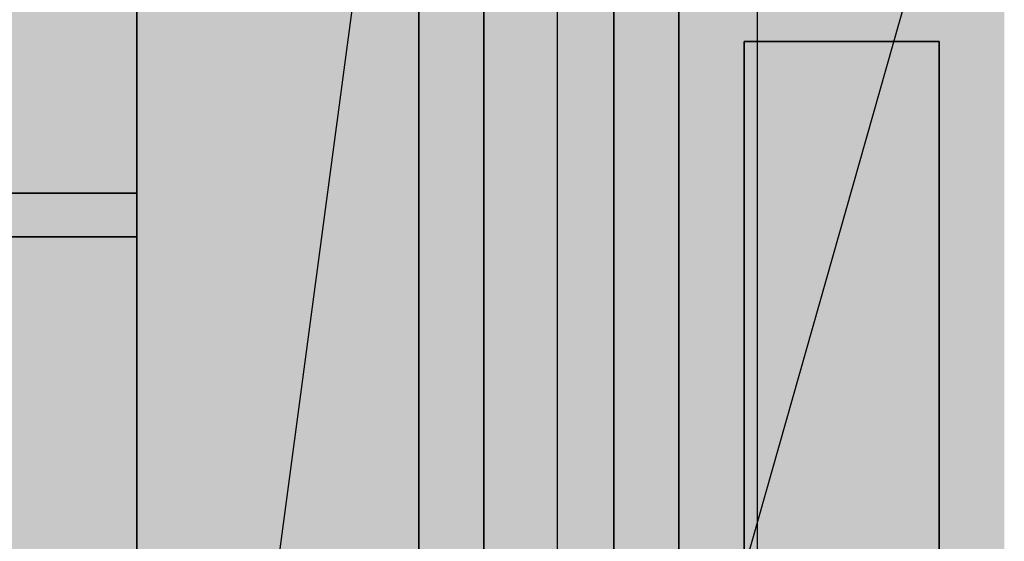
# Model space of a CAD drawing. Units: millimetres. Extents: x 130 to 1021, y 147 to 699.
# Tile 28 of 40: x 442 to 487, y 524 to 548. Entities that reach past the tile are written whole.
import ezdxf

# ---------------------------------------------------------------- set-up
doc = ezdxf.new("R2010")
doc.units = ezdxf.units.MM
doc.header["$MEASUREMENT"] = 0
for name, color, linetype, lineweight in [('A-ANNO-DIMS', 2, 'Continuous', 18), ('A-ELEV', 7, 'Continuous', 35), ('A-ELEV-PATT', 9, 'Continuous', 13)]:
    doc.layers.add(name, color=color, linetype=linetype, lineweight=lineweight)
doc.styles.get("Standard").update_dxf_attribs({"font": 'arial.ttf'})
doc.dimstyles.get("Standard").update_dxf_attribs({"dimtxt": 20, "dimasz": 10, "dimexe": 10, "dimexo": 10, "dimgap": 5, "dimtad": 0, "dimtih": 1, "dimtoh": 1, "dimdec": 0, "dimzin": 0, "dimdsep": 46, "dimtxsty": 'Standard', "dimcen": 5, "dimadec": 0, "dimazin": 0, "dimtfac": 1, "dimtdec": 0, "dimtofl": 0, "dimtmove": 0, "dimatfit": 3, "dimfxl": 1, "dimtolj": 1, "dimtzin": 0, "dimarcsym": 0})

# ---------------------------------------------------------------- blocks, each defined once
blk = doc.blocks.new('*D11')
at = {"layer": 'A-ANNO-DIMS', "color": 0, "lineweight": -2, "transparency": 16777216}
for p, q in [((737.374, 648.699), (737.374, 149.739)), ((299.374, 566.947), (299.374, 149.739)), ((309.374, 159.739), (490.857, 159.739)), ((727.374, 159.739), (545.891, 159.739))]:
    blk.add_line(p, q, dxfattribs=at)
at = {"layer": 'A-ANNO-DIMS', "color": 0, "transparency": 16777216}
for points in [[(309.374, 161.406), (309.374, 158.073), (299.374, 159.739)], [(727.374, 161.406), (727.374, 158.073), (737.374, 159.739)]]:
    blk.add_solid(points, dxfattribs=at)
at = {"layer": 'Defpoints', "color": 0, "transparency": 16777216}
for p in [(737.374, 658.699), (299.374, 576.947), (737.374, 159.739)]:
    blk.add_point(p, dxfattribs=at)
at = {"layer": 'A-ANNO-DIMS', "color": 0, "transparency": 16777216, "insert": (518.374, 159.739), "char_height": 20, "attachment_point": 5}
blk.add_mtext('\\A1;438', dxfattribs=at)
blk = doc.blocks.new('*D12')
at = {"layer": 'A-ANNO-DIMS', "color": 0, "lineweight": -2, "transparency": 16777216}
for p, q in [((477.374, 661.947), (265.074, 661.947)), ((275.074, 651.947), (275.074, 438.205)), ((275.074, 194.039), (275.074, 407.782)), ((357.163, 184.039), (265.074, 184.039))]:
    blk.add_line(p, q, dxfattribs=at)
at = {"layer": 'A-ANNO-DIMS', "color": 0, "transparency": 16777216}
for points in [[(273.407, 651.947), (276.74, 651.947), (275.074, 661.947)], [(273.407, 194.039), (276.74, 194.039), (275.074, 184.039)]]:
    blk.add_solid(points, dxfattribs=at)
at = {"layer": 'Defpoints', "color": 0, "transparency": 16777216}
for p in [(275.074, 661.947), (487.374, 661.947), (367.163, 184.039)]:
    blk.add_point(p, dxfattribs=at)
at = {"layer": 'A-ANNO-DIMS', "color": 0, "transparency": 16777216, "insert": (275.074, 422.993), "char_height": 20, "attachment_point": 5}
blk.add_mtext('\\A1;477.9', dxfattribs=at)
blk = doc.blocks.new('*D16')
at = {"layer": 'A-ANNO-DIMS', "color": 0, "lineweight": -2, "transparency": 16777216}
for p, q in [((357.941, 411.947), (357.941, 696.247)), ((363.922, 579.884), (363.922, 696.247)), ((347.941, 686.247), (337.941, 686.247)), ((373.922, 686.247), (383.922, 686.247))]:
    blk.add_line(p, q, dxfattribs=at)
at = {"layer": 'A-ANNO-DIMS', "color": 0, "transparency": 16777216}
for points in [[(347.941, 687.914), (347.941, 684.581), (357.941, 686.247)], [(373.922, 687.914), (373.922, 684.581), (363.922, 686.247)]]:
    blk.add_solid(points, dxfattribs=at)
at = {"layer": 'Defpoints', "color": 0, "transparency": 16777216}
for p in [(363.922, 686.247), (363.922, 569.884), (357.941, 401.947)]:
    blk.add_point(p, dxfattribs=at)
at = {"layer": 'A-ANNO-DIMS', "color": 0, "transparency": 16777216, "insert": (420.737, 686.247), "char_height": 20, "attachment_point": 5}
blk.add_mtext('\\A1;5.981', dxfattribs=at)
blk = doc.blocks.new('*D17')
at = {"layer": 'A-ANNO-DIMS', "color": 0, "lineweight": -2, "transparency": 16777216}
for p, q in [((363.922, 579.884), (363.922, 696.247)), ((375.85, 490.216), (375.85, 696.247)), ((353.922, 686.247), (343.922, 686.247)), ((385.85, 686.247), (395.85, 686.247))]:
    blk.add_line(p, q, dxfattribs=at)
at = {"layer": 'A-ANNO-DIMS', "color": 0, "transparency": 16777216}
for points in [[(353.922, 687.914), (353.922, 684.581), (363.922, 686.247)], [(385.85, 687.914), (385.85, 684.581), (375.85, 686.247)]]:
    blk.add_solid(points, dxfattribs=at)
at = {"layer": 'Defpoints', "color": 0, "transparency": 16777216}
for p in [(375.85, 686.247), (363.922, 569.884), (375.85, 480.216)]:
    blk.add_point(p, dxfattribs=at)
at = {"layer": 'A-ANNO-DIMS', "color": 0, "transparency": 16777216, "insert": (441.444, 686.247), "char_height": 20, "attachment_point": 5}
blk.add_mtext('\\A1;11.928', dxfattribs=at)
blk = doc.blocks.new('*D18')
at = {"layer": 'A-ANNO-DIMS', "color": 0, "lineweight": -2, "transparency": 16777216}
for p, q in [((375.85, 490.216), (375.85, 696.247)), ((382.374, 388.947), (382.374, 696.247)), ((365.85, 686.247), (355.85, 686.247)), ((392.374, 686.247), (402.374, 686.247))]:
    blk.add_line(p, q, dxfattribs=at)
at = {"layer": 'A-ANNO-DIMS', "color": 0, "transparency": 16777216}
for points in [[(365.85, 687.914), (365.85, 684.581), (375.85, 686.247)], [(392.374, 687.914), (392.374, 684.581), (382.374, 686.247)]]:
    blk.add_solid(points, dxfattribs=at)
at = {"layer": 'Defpoints', "color": 0, "transparency": 16777216}
for p in [(382.374, 686.247), (375.85, 480.216), (382.374, 378.947)]:
    blk.add_point(p, dxfattribs=at)
at = {"layer": 'A-ANNO-DIMS', "color": 0, "transparency": 16777216, "insert": (441.132, 686.247), "char_height": 20, "attachment_point": 5}
blk.add_mtext('\\A1;6.524', dxfattribs=at)
blk = doc.blocks.new('*D19')
at = {"layer": 'A-ANNO-DIMS', "color": 0, "lineweight": -2, "transparency": 16777216}
for p, q in [((382.374, 388.947), (382.374, 696.247)), ((414.652, 510.881), (414.652, 696.247)), ((392.374, 686.247), (404.652, 686.247)), ((414.652, 686.247), (424.652, 686.247))]:
    blk.add_line(p, q, dxfattribs=at)
at = {"layer": 'A-ANNO-DIMS', "color": 0, "transparency": 16777216}
for points in [[(392.374, 687.914), (392.374, 684.581), (382.374, 686.247)], [(404.652, 687.914), (404.652, 684.581), (414.652, 686.247)]]:
    blk.add_solid(points, dxfattribs=at)
at = {"layer": 'Defpoints', "color": 0, "transparency": 16777216}
for p in [(414.652, 686.247), (414.652, 500.881), (382.374, 378.947)]:
    blk.add_point(p, dxfattribs=at)
at = {"layer": 'A-ANNO-DIMS', "color": 0, "transparency": 16777216, "insert": (463.411, 686.247), "char_height": 20, "attachment_point": 5}
blk.add_mtext('\\A1;32.28', dxfattribs=at)
blk = doc.blocks.new('*D20')
at = {"layer": 'A-ANNO-DIMS', "color": 0, "lineweight": -2, "transparency": 16777216}
for p, q in [((414.652, 510.881), (414.652, 696.247)), ((432.374, 388.947), (432.374, 696.247)), ((404.652, 686.247), (394.652, 686.247)), ((442.374, 686.247), (452.374, 686.247))]:
    blk.add_line(p, q, dxfattribs=at)
at = {"layer": 'A-ANNO-DIMS', "color": 0, "transparency": 16777216}
for points in [[(404.652, 687.914), (404.652, 684.581), (414.652, 686.247)], [(442.374, 687.914), (442.374, 684.581), (432.374, 686.247)]]:
    blk.add_solid(points, dxfattribs=at)
at = {"layer": 'Defpoints', "color": 0, "transparency": 16777216}
for p in [(432.374, 686.247), (414.652, 500.881), (432.374, 378.947)]:
    blk.add_point(p, dxfattribs=at)
at = {"layer": 'A-ANNO-DIMS', "color": 0, "transparency": 16777216, "insert": (490.075, 686.247), "char_height": 20, "attachment_point": 5}
blk.add_mtext('\\A1;17.72', dxfattribs=at)
blk = doc.blocks.new('*D21')
at = {"layer": 'A-ANNO-DIMS', "color": 0, "lineweight": -2, "transparency": 16777216}
for p, q in [((432.374, 388.947), (432.374, 696.247)), ((447.374, 656.947), (447.374, 696.247)), ((422.374, 686.247), (412.374, 686.247)), ((457.374, 686.247), (467.374, 686.247))]:
    blk.add_line(p, q, dxfattribs=at)
at = {"layer": 'A-ANNO-DIMS', "color": 0, "transparency": 16777216}
for points in [[(422.374, 687.914), (422.374, 684.581), (432.374, 686.247)], [(457.374, 687.914), (457.374, 684.581), (447.374, 686.247)]]:
    blk.add_solid(points, dxfattribs=at)
at = {"layer": 'Defpoints', "color": 0, "transparency": 16777216}
for p in [(447.374, 686.247), (447.374, 646.947), (432.374, 378.947)]:
    blk.add_point(p, dxfattribs=at)
at = {"layer": 'A-ANNO-DIMS', "color": 0, "transparency": 16777216, "insert": (485.832, 686.247), "char_height": 20, "attachment_point": 5}
blk.add_mtext('\\A1;15', dxfattribs=at)
blk = doc.blocks.new('*D22')
at = {"layer": 'A-ANNO-DIMS', "color": 0, "lineweight": -2, "transparency": 16777216}
for p, q in [((447.374, 656.947), (447.374, 696.247)), ((466.767, 403.947), (466.767, 696.247)), ((437.374, 686.247), (427.374, 686.247)), ((476.767, 686.247), (486.767, 686.247))]:
    blk.add_line(p, q, dxfattribs=at)
at = {"layer": 'A-ANNO-DIMS', "color": 0, "transparency": 16777216}
for points in [[(437.374, 687.914), (437.374, 684.581), (447.374, 686.247)], [(476.767, 687.914), (476.767, 684.581), (466.767, 686.247)]]:
    blk.add_solid(points, dxfattribs=at)
at = {"layer": 'Defpoints', "color": 0, "transparency": 16777216}
for p in [(466.767, 686.247), (447.374, 646.947), (466.767, 393.947)]:
    blk.add_point(p, dxfattribs=at)
at = {"layer": 'A-ANNO-DIMS', "color": 0, "transparency": 16777216, "insert": (532.34, 686.247), "char_height": 20, "attachment_point": 5}
blk.add_mtext('\\A1;19.393', dxfattribs=at)
blk = doc.blocks.new('*D23')
at = {"layer": 'A-ANNO-DIMS', "color": 0, "lineweight": -2, "transparency": 16777216}
for p, q in [((466.767, 403.947), (466.767, 696.247)), ((475.988, 209.039), (475.988, 696.247)), ((456.767, 686.247), (446.767, 686.247)), ((485.988, 686.247), (495.988, 686.247))]:
    blk.add_line(p, q, dxfattribs=at)
at = {"layer": 'A-ANNO-DIMS', "color": 0, "transparency": 16777216}
for points in [[(456.767, 687.914), (456.767, 684.581), (466.767, 686.247)], [(485.988, 687.914), (485.988, 684.581), (475.988, 686.247)]]:
    blk.add_solid(points, dxfattribs=at)
at = {"layer": 'Defpoints', "color": 0, "transparency": 16777216}
for p in [(475.988, 686.247), (466.767, 393.947), (475.988, 199.039)]:
    blk.add_point(p, dxfattribs=at)
at = {"layer": 'A-ANNO-DIMS', "color": 0, "transparency": 16777216, "insert": (534.631, 686.247), "char_height": 20, "attachment_point": 5}
blk.add_mtext('\\A1;9.222', dxfattribs=at)
blk = doc.blocks.new('*D24')
at = {"layer": 'A-ANNO-DIMS', "color": 0, "lineweight": -2, "transparency": 16777216}
for p, q in [((475.988, 209.039), (475.988, 696.247)), ((487.374, 671.947), (487.374, 696.247)), ((465.988, 686.247), (455.988, 686.247)), ((497.374, 686.247), (507.374, 686.247))]:
    blk.add_line(p, q, dxfattribs=at)
at = {"layer": 'A-ANNO-DIMS', "color": 0, "transparency": 16777216}
for points in [[(465.988, 687.914), (465.988, 684.581), (475.988, 686.247)], [(497.374, 687.914), (497.374, 684.581), (487.374, 686.247)]]:
    blk.add_solid(points, dxfattribs=at)
at = {"layer": 'Defpoints', "color": 0, "transparency": 16777216}
for p in [(487.374, 686.247), (487.374, 661.947), (475.988, 199.039)]:
    blk.add_point(p, dxfattribs=at)
at = {"layer": 'A-ANNO-DIMS', "color": 0, "transparency": 16777216, "insert": (553.022, 686.247), "char_height": 20, "attachment_point": 5}
blk.add_mtext('\\A1;11.385', dxfattribs=at)
blk = doc.blocks.new('*D25')
at = {"layer": 'A-ANNO-DIMS', "color": 0, "lineweight": -2, "transparency": 16777216}
for p, q in [((487.374, 671.947), (487.374, 696.247)), ((494.102, 506.908), (494.102, 696.247)), ((477.374, 686.247), (467.374, 686.247)), ((504.102, 686.247), (514.102, 686.247))]:
    blk.add_line(p, q, dxfattribs=at)
at = {"layer": 'A-ANNO-DIMS', "color": 0, "transparency": 16777216}
for points in [[(477.374, 687.914), (477.374, 684.581), (487.374, 686.247)], [(504.102, 687.914), (504.102, 684.581), (494.102, 686.247)]]:
    blk.add_solid(points, dxfattribs=at)
at = {"layer": 'Defpoints', "color": 0, "transparency": 16777216}
for p in [(494.102, 686.247), (487.374, 661.947), (494.102, 496.908)]:
    blk.add_point(p, dxfattribs=at)
at = {"layer": 'A-ANNO-DIMS', "color": 0, "transparency": 16777216, "insert": (552.922, 686.247), "char_height": 20, "attachment_point": 5}
blk.add_mtext('\\A1;6.728', dxfattribs=at)
blk = doc.blocks.new('*D26')
at = {"layer": 'A-ANNO-DIMS', "color": 0, "lineweight": -2, "transparency": 16777216}
for p, q in [((494.102, 506.908), (494.102, 696.247)), ((502.374, 593.947), (502.374, 696.247)), ((484.102, 686.247), (474.102, 686.247)), ((512.374, 686.247), (522.374, 686.247))]:
    blk.add_line(p, q, dxfattribs=at)
at = {"layer": 'A-ANNO-DIMS', "color": 0, "transparency": 16777216}
for points in [[(484.102, 687.914), (484.102, 684.581), (494.102, 686.247)], [(512.374, 687.914), (512.374, 684.581), (502.374, 686.247)]]:
    blk.add_solid(points, dxfattribs=at)
at = {"layer": 'Defpoints', "color": 0, "transparency": 16777216}
for p in [(502.374, 686.247), (502.374, 583.947), (494.102, 496.908)]:
    blk.add_point(p, dxfattribs=at)
at = {"layer": 'A-ANNO-DIMS', "color": 0, "transparency": 16777216, "insert": (561.03, 686.247), "char_height": 20, "attachment_point": 5}
blk.add_mtext('\\A1;8.272', dxfattribs=at)
blk = doc.blocks.new('*D69')
at = {"layer": 'A-ANNO-DIMS', "color": 0, "lineweight": -2, "transparency": 16777216}
for p, q in [((507.746, 572.261), (483.091, 501.813)), ((517.746, 572.261), (507.746, 572.261)), ((433.191, 354.23), (433.191, 364.23)), ((428.191, 359.23), (438.191, 359.23))]:
    blk.add_line(p, q, dxfattribs=at)
at = {"layer": 'A-ANNO-DIMS', "color": 0, "transparency": 16777216}
blk.add_solid([(481.518, 502.363), (484.664, 501.262), (479.788, 492.374)], dxfattribs=at)
at = {"layer": 'Defpoints', "color": 0, "transparency": 16777216}
for p in [(479.788, 492.374), (433.191, 359.23)]:
    blk.add_point(p, dxfattribs=at)
at = {"layer": 'A-ANNO-DIMS', "color": 0, "transparency": 16777216, "insert": (573.824, 572.261), "char_height": 20, "attachment_point": 5}
blk.add_mtext('\\A1;R141.06', dxfattribs=at)
blk = doc.blocks.new('*D71')
at = {"layer": 'A-ANNO-DIMS', "color": 0, "lineweight": -2, "transparency": 16777216}
for p, q in [((492.108, 581.609), (472.542, 512.666)), ((502.108, 581.609), (492.108, 581.609)), ((432.65, 367.109), (432.65, 377.109)), ((427.65, 372.109), (437.65, 372.109))]:
    blk.add_line(p, q, dxfattribs=at)
at = {"layer": 'A-ANNO-DIMS', "color": 0, "transparency": 16777216}
blk.add_solid([(470.938, 513.121), (474.145, 512.211), (469.812, 503.046)], dxfattribs=at)
at = {"layer": 'Defpoints', "color": 0, "transparency": 16777216}
for p in [(469.812, 503.046), (432.65, 372.109)]:
    blk.add_point(p, dxfattribs=at)
at = {"layer": 'A-ANNO-DIMS', "color": 0, "transparency": 16777216, "insert": (548.493, 581.609), "char_height": 20, "attachment_point": 5}
blk.add_mtext('\\A1;R136.1', dxfattribs=at)
blk = doc.blocks.new('*D72')
at = {"layer": 'A-ANNO-DIMS', "color": 0, "lineweight": -2, "transparency": 16777216}
for p, q in [((460.658, 573.64), (451.279, 503.49)), ((470.658, 573.64), (460.658, 573.64)), ((432.115, 355.142), (432.115, 365.142)), ((427.115, 360.142), (437.115, 360.142))]:
    blk.add_line(p, q, dxfattribs=at)
at = {"layer": 'A-ANNO-DIMS', "color": 0, "transparency": 16777216}
blk.add_solid([(449.628, 503.711), (452.931, 503.27), (449.954, 493.579)], dxfattribs=at)
at = {"layer": 'Defpoints', "color": 0, "transparency": 16777216}
for p in [(449.954, 493.579), (432.115, 360.142)]:
    blk.add_point(p, dxfattribs=at)
at = {"layer": 'A-ANNO-DIMS', "color": 0, "transparency": 16777216, "insert": (526.64, 573.64), "char_height": 20, "attachment_point": 5}
blk.add_mtext('\\A1;R134.62', dxfattribs=at)

msp = doc.modelspace()

# ---------------------------------------------------------------- hatches: boundary and pattern name
at = {"layer": 'A-ELEV-PATT'}
h = msp.add_hatch(color=256, dxfattribs=at)
h.dxf.hatch_style = 1
h.paths.add_polyline_path([(737.3738, 658.6988, 0.0135961), (632.4019, 661.9473), (607.3738, 661.9473), (487.3738, 661.9473), (487.3738, 649.9473), (607.3738, 649.9473), (632.3794, 649.9473, -0.0136841), (737.3738, 646.6784)])
h.paths.add_polyline_path([(732.3738, 643.9599, 0.0130529), (632.3738, 646.9473), (607.3738, 646.9473), (487.3738, 646.9473), (487.3738, 596.9473), (632.3738, 596.9473, -0.0130529), (732.3738, 593.9599)])
h.paths.add_polyline_path([(737.3738, 593.6732, 0.0137063), (632.3738, 596.9473), (487.3738, 596.9473), (487.3738, 586.9473), (632.355, 586.9473, -0.0137808), (737.3738, 583.6559)])
h.paths.add_polyline_path([(447.3738, 646.9473), (307.3738, 646.9473), (302.3738, 646.9473), (302.3738, 634.9473), (447.3738, 634.9473)])
h.paths.add_polyline_path([(447.3738, 631.9473), (307.3738, 631.9473), (307.3738, 586.9473), (447.3738, 586.9473)])
h.paths.add_polyline_path([(447.3738, 586.9473), (307.3738, 586.9473), (302.3738, 586.9473), (302.3738, 576.9473), (447.3738, 576.9473)])
h.paths.add_polyline_path([(447.3738, 573.9473), (367.3738, 573.9473), (367.3738, 539.9473), (447.3738, 539.9473)])
h.paths.add_polyline_path([(447.3738, 537.9473), (367.3738, 537.9473), (367.3738, 507.9473), (400.392, 507.4253, -0.001728), (401.3281, 507.6451, -0.5220025), (425.6117, 511.0391, -0.0391849), (447.3738, 510.4359), (447.3738, 510.7883)])
h.paths.add_polyline_path([(394.7238, 505.9473), (367.3738, 505.9473), (367.3738, 476.9473, -0.0146512), (375.8501, 480.2159), (376.1506, 499.2266, -0.0355419)])
h.paths.add_polyline_path([(632.3738, 583.9473), (552.3738, 583.9473), (552.3738, 550.9473), (632.3738, 550.9473)])
h.paths.add_polyline_path([(632.3738, 548.9473), (552.3738, 548.9473), (552.3738, 515.9473), (632.3738, 515.9473)])
h.paths.add_polyline_path([(632.3738, 513.9473), (552.3738, 513.9473), (552.3738, 476.9473), (632.3738, 476.9473)])
h.paths.add_polyline_path([(737.3738, 473.6903, 0.0136326), (632.3926, 476.9473), (552.3738, 476.9473), (487.3738, 476.9473), (487.3738, 466.9473), (632.3738, 466.9473, -0.0137063), (737.3738, 463.6732)])
h.paths.add_polyline_path([(732.3738, 460.9552, 0.0130741), (632.3681, 463.9473), (487.3738, 463.9473), (487.3738, 407.735, -0.0032286), (489.3544, 406.9473), (632.3926, 406.9473, -0.0129826), (732.3738, 403.9755)])
h.paths.add_polyline_path([(487.3738, 463.9473, 0.20133), (367.3738, 463.9473), (367.3738, 407.735, -0.1882031), (487.3738, 407.735)])
h.paths.add_polyline_path([(367.3738, 476.9473), (367.3738, 466.9473, -0.2013309), (487.3738, 466.9473), (487.3738, 476.9473, 0.20133)])
h.paths.add_polyline_path([(367.3738, 463.9473), (307.3738, 463.9473), (307.3738, 401.9473), (357.9413, 401.9473), (367.3738, 407.735)])
h.paths.add_polyline_path([(367.3738, 476.9473), (302.3738, 476.9473), (302.3738, 466.9473), (367.3738, 466.9473)])
h.paths.add_polyline_path([(632.8184, 366.9453), (552.3738, 366.9453), (552.3738, 393.9473), (632.8184, 393.9473)])
h.paths.add_polyline_path([(632.8184, 357.2114), (632.8184, 363.9453), (552.3738, 363.9453), (552.3738, 357.2114), (552.3738, 336.9453), (632.8184, 336.9453)])
h.paths.add_polyline_path([(632.8184, 333.9453), (552.3738, 333.9453), (552.3738, 306.9453), (632.8184, 306.9453)])
h.paths.add_polyline_path([(632.8184, 303.9453), (552.3738, 303.9453), (552.3738, 273.9473), (632.355, 273.9473, 0.0000608), (632.8184, 273.9491)])
h.paths.add_polyline_path([(737.3738, 403.6903, 0.0136326), (632.3926, 406.9473), (489.3544, 406.9473, 0.1915481), (367.3738, 407.735), (367.3738, 396.9473, -0.2013309), (487.3738, 396.9473), (632.3738, 396.9473, -0.0137063), (737.3738, 393.6732)])
h.paths.add_polyline_path([(357.9413, 401.9473), (307.3738, 401.9473), (307.3738, 391.9473), (357.9413, 391.9473)])
h.paths.add_polyline_path([(357.9413, 357.2114), (357.9413, 388.9473), (307.3738, 388.9473), (307.3738, 357.2114), (307.3738, 273.9473), (357.9413, 273.9473)])
h.paths.add_polyline_path([(732.3738, 263.93, -0.0130317), (632.3794, 260.9473), (466.7667, 260.9473), (466.7667, 240.9473), (469.8406, 236.978), (469.8406, 221.978), (472.9145, 218.0087), (472.9145, 213.9473), (607.3738, 213.9473), (732.3738, 213.9473)])
h.paths.add_polyline_path([(732.3738, 290.889), (722.479, 290.889), (722.479, 301.889), (732.3738, 301.889), (732.3738, 305.889), (722.479, 305.889), (722.479, 316.889), (732.3738, 316.889), (732.3738, 320.889), (722.479, 320.889), (722.479, 331.889), (732.3738, 331.889), (732.3738, 335.889), (722.479, 335.889), (722.479, 346.889), (732.3738, 346.889), (732.3738, 350.889), (722.479, 350.889), (722.479, 361.889), (732.3738, 361.889), (732.3738, 365.889), (722.479, 365.889), (722.479, 376.889), (732.3738, 376.889), (732.3738, 380.889), (722.479, 380.889), (722.479, 391.4848, 0.0005233), (718.479, 391.6843), (718.479, 380.889), (707.479, 380.889), (707.479, 392.1896, 0.0005231), (703.479, 392.3576), (703.479, 380.889), (692.479, 380.889), (692.479, 392.7765, 0.0005229), (688.479, 392.9131), (688.479, 380.889), (677.479, 380.889), (677.479, 393.2456, 0.0005228), (673.479, 393.3508), (673.479, 380.889), (662.479, 380.889), (662.479, 393.597, 0.0005227), (658.479, 393.6709), (658.479, 380.889), (647.479, 380.889), (647.479, 393.8308, 0.0005226), (643.479, 393.8732), (643.479, 380.889), (632.8184, 380.889), (632.8184, 376.889), (643.479, 376.889), (643.479, 365.889), (632.8184, 365.889), (632.8184, 361.889), (643.479, 361.889), (643.479, 350.889), (632.8184, 350.889), (632.8184, 346.889), (643.479, 346.889), (643.479, 335.889), (632.8184, 335.889), (632.8184, 331.889), (643.479, 331.889), (643.479, 320.889), (632.8184, 320.889), (632.8184, 316.889), (643.479, 316.889), (643.479, 305.889), (632.8184, 305.889), (632.8184, 301.889), (643.479, 301.889), (643.479, 290.889), (632.8184, 290.889), (632.8184, 286.889), (643.479, 286.889), (643.479, 274.0217, 0.0005246), (647.479, 274.0643), (647.479, 286.889), (658.479, 286.889), (658.479, 274.2248, 0.0005246), (662.479, 274.2989), (662.479, 286.889), (673.479, 286.889), (673.479, 274.546, 0.0005247), (677.479, 274.6516), (677.479, 286.889), (688.479, 286.889), (688.479, 274.9853, 0.0005248), (692.479, 275.1224), (692.479, 286.889), (703.479, 286.889), (703.479, 275.5429, 0.000525), (707.479, 275.7115), (707.479, 286.889), (718.479, 286.889), (718.479, 276.2187, 0.0005252), (722.479, 276.4189), (722.479, 286.889), (732.3738, 286.889)])
h.paths.add_polyline_path([(718.479, 290.889), (707.479, 290.889), (707.479, 301.889), (718.479, 301.889)], flags=16)
h.paths.add_polyline_path([(703.479, 290.889), (692.479, 290.889), (692.479, 301.889), (703.479, 301.889)], flags=16)
h.paths.add_polyline_path([(718.479, 305.889), (707.479, 305.889), (707.479, 316.889), (718.479, 316.889)], flags=16)
h.paths.add_polyline_path([(703.479, 305.889), (692.479, 305.889), (692.479, 316.889), (703.479, 316.889)], flags=16)
h.paths.add_polyline_path([(688.479, 290.889), (677.479, 290.889), (677.479, 301.889), (688.479, 301.889)], flags=16)
h.paths.add_polyline_path([(718.479, 320.889), (707.479, 320.889), (707.479, 331.889), (718.479, 331.889)], flags=16)
h.paths.add_polyline_path([(688.479, 305.889), (677.479, 305.889), (677.479, 316.889), (688.479, 316.889)], flags=16)
h.paths.add_polyline_path([(703.479, 320.889), (692.479, 320.889), (692.479, 331.889), (703.479, 331.889)], flags=16)
h.paths.add_polyline_path([(688.479, 320.889), (677.479, 320.889), (677.479, 331.889), (688.479, 331.889)], flags=16)
h.paths.add_polyline_path([(673.479, 290.889), (662.479, 290.889), (662.479, 301.889), (673.479, 301.889)], flags=16)
h.paths.add_polyline_path([(718.479, 335.889), (707.479, 335.889), (707.479, 346.889), (718.479, 346.889)], flags=16)
h.paths.add_polyline_path([(673.479, 305.889), (662.479, 305.889), (662.479, 316.889), (673.479, 316.889)], flags=16)
h.paths.add_polyline_path([(703.479, 335.889), (692.479, 335.889), (692.479, 346.889), (703.479, 346.889)], flags=16)
h.paths.add_polyline_path([(673.479, 320.889), (662.479, 320.889), (662.479, 331.889), (673.479, 331.889)], flags=16)
h.paths.add_polyline_path([(688.479, 335.889), (677.479, 335.889), (677.479, 346.889), (688.479, 346.889)], flags=16)
h.paths.add_polyline_path([(658.479, 290.889), (647.479, 290.889), (647.479, 301.889), (658.479, 301.889)], flags=16)
h.paths.add_polyline_path([(718.479, 350.889), (707.479, 350.889), (707.479, 361.889), (718.479, 361.889)], flags=16)
h.paths.add_polyline_path([(658.479, 305.889), (647.479, 305.889), (647.479, 316.889), (658.479, 316.889)], flags=16)
h.paths.add_polyline_path([(703.479, 350.889), (692.479, 350.889), (692.479, 361.889), (703.479, 361.889)], flags=16)
h.paths.add_polyline_path([(673.479, 335.889), (662.479, 335.889), (662.479, 346.889), (673.479, 346.889)], flags=16)
h.paths.add_polyline_path([(658.479, 320.889), (647.479, 320.889), (647.479, 331.889), (658.479, 331.889)], flags=16)
h.paths.add_polyline_path([(688.479, 350.889), (677.479, 350.889), (677.479, 361.889), (688.479, 361.889)], flags=16)
h.paths.add_polyline_path([(718.479, 365.889), (707.479, 365.889), (707.479, 376.889), (718.479, 376.889)], flags=16)
h.paths.add_polyline_path([(658.479, 335.889), (647.479, 335.889), (647.479, 346.889), (658.479, 346.889)], flags=16)
h.paths.add_polyline_path([(673.479, 350.889), (662.479, 350.889), (662.479, 361.889), (673.479, 361.889)], flags=16)
h.paths.add_polyline_path([(703.479, 365.889), (692.479, 365.889), (692.479, 376.889), (703.479, 376.889)], flags=16)
h.paths.add_polyline_path([(688.479, 365.889), (677.479, 365.889), (677.479, 376.889), (688.479, 376.889)], flags=16)
h.paths.add_polyline_path([(658.479, 350.889), (647.479, 350.889), (647.479, 361.889), (658.479, 361.889)], flags=16)
h.paths.add_polyline_path([(673.479, 365.889), (662.479, 365.889), (662.479, 376.889), (673.479, 376.889)], flags=16)
h.paths.add_polyline_path([(658.479, 365.889), (647.479, 365.889), (647.479, 376.889), (658.479, 376.889)], flags=16)
h.paths.add_polyline_path([(732.3738, 503.9786), (722.3392, 503.9786), (722.3392, 514.9786), (732.3738, 514.9786), (732.3738, 518.9786), (722.3392, 518.9786), (722.3392, 529.9786), (732.3738, 529.9786), (732.3738, 533.9786), (722.3392, 533.9786), (722.3392, 544.9786), (732.3738, 544.9786), (732.3738, 546.9473), (732.3738, 548.9786), (722.3392, 548.9786), (722.3392, 559.9786), (732.3738, 559.9786), (732.3738, 563.9786), (722.3392, 563.9786), (722.3392, 574.9786), (732.3738, 574.9786), (732.3738, 578.9786), (722.3392, 578.9786), (722.3392, 581.4789, 0.000526), (718.3392, 581.6791), (718.3392, 578.9786), (707.3392, 578.9786), (707.3392, 582.1863, 0.0005258), (703.3392, 582.355), (703.3392, 578.9786), (692.3392, 578.9786), (692.3392, 582.7752, 0.0005257), (688.3392, 582.9123), (688.3392, 578.9786), (677.3392, 578.9786), (677.3392, 583.2457, 0.0005255), (673.3392, 583.3512), (673.3392, 578.9786), (662.3392, 578.9786), (662.3392, 583.5978, 0.0005254), (658.3392, 583.6718), (658.3392, 578.9786), (647.3392, 578.9786), (647.3392, 583.8317, 0.0005254), (643.3392, 583.8741), (643.3392, 578.9786), (632.3738, 578.9786), (632.3738, 574.9786), (643.3392, 574.9786), (643.3392, 563.9786), (632.3738, 563.9786), (632.3738, 559.9786), (643.3392, 559.9786), (643.3392, 548.9786), (632.3738, 548.9786), (632.3738, 544.9786), (643.3392, 544.9786), (643.3392, 533.9786), (632.3738, 533.9786), (632.3738, 529.9786), (643.3392, 529.9786), (643.3392, 518.9786), (632.3738, 518.9786), (632.3738, 515.9473), (632.3738, 514.9786), (643.3392, 514.9786), (643.3392, 503.9786), (632.3738, 503.9786), (632.3738, 499.9786), (643.3392, 499.9786), (643.3392, 488.9786), (632.3738, 488.9786), (632.3738, 484.9786), (643.3392, 484.9786), (643.3392, 476.8751, -0.0005191), (647.3392, 476.8332), (647.3392, 484.9786), (658.3392, 484.9786), (658.3392, 476.6752, -0.0005192), (662.3392, 476.6022), (662.3392, 484.9786), (673.3392, 484.9786), (673.3392, 476.3585, -0.0005193), (677.3392, 476.2543), (677.3392, 484.9786), (688.3392, 484.9786), (688.3392, 475.9248, -0.0005194), (692.3392, 475.7894), (692.3392, 484.9786), (703.3392, 484.9786), (703.3392, 475.3741, -0.0005195), (707.3392, 475.2075), (707.3392, 484.9786), (718.3392, 484.9786), (718.3392, 474.7064, -0.0005197), (722.3392, 474.5086), (722.3392, 484.9786), (732.3738, 484.9786), (732.3738, 488.9786), (722.3392, 488.9786), (722.3392, 499.9786), (732.3738, 499.9786)])
h.paths.add_polyline_path([(718.3392, 503.9786), (707.3392, 503.9786), (707.3392, 514.9786), (718.3392, 514.9786)], flags=16)
h.paths.add_polyline_path([(718.3392, 499.9786), (718.3392, 488.9786), (707.3392, 488.9786), (707.3392, 499.9786)], flags=16)
h.paths.add_polyline_path([(718.3392, 518.9786), (707.3392, 518.9786), (707.3392, 529.9786), (718.3392, 529.9786)], flags=16)
h.paths.add_polyline_path([(703.3392, 503.9786), (692.3392, 503.9786), (692.3392, 514.9786), (703.3392, 514.9786)], flags=16)
h.paths.add_polyline_path([(703.3392, 499.9786), (703.3392, 488.9786), (692.3392, 488.9786), (692.3392, 499.9786)], flags=16)
h.paths.add_polyline_path([(703.3392, 518.9786), (692.3392, 518.9786), (692.3392, 529.9786), (703.3392, 529.9786)], flags=16)
h.paths.add_polyline_path([(718.3392, 533.9786), (707.3392, 533.9786), (707.3392, 544.9786), (718.3392, 544.9786)], flags=16)
h.paths.add_polyline_path([(688.3392, 503.9786), (677.3392, 503.9786), (677.3392, 514.9786), (688.3392, 514.9786)], flags=16)
h.paths.add_polyline_path([(688.3392, 499.9786), (688.3392, 488.9786), (677.3392, 488.9786), (677.3392, 499.9786)], flags=16)
h.paths.add_polyline_path([(703.3392, 533.9786), (692.3392, 533.9786), (692.3392, 544.9786), (703.3392, 544.9786)], flags=16)
h.paths.add_polyline_path([(688.3392, 518.9786), (677.3392, 518.9786), (677.3392, 529.9786), (688.3392, 529.9786)], flags=16)
h.paths.add_polyline_path([(688.3392, 533.9786), (677.3392, 533.9786), (677.3392, 544.9786), (688.3392, 544.9786)], flags=16)
h.paths.add_polyline_path([(718.3392, 548.9786), (707.3392, 548.9786), (707.3392, 559.9786), (718.3392, 559.9786)], flags=16)
h.paths.add_polyline_path([(673.3392, 503.9786), (662.3392, 503.9786), (662.3392, 514.9786), (673.3392, 514.9786)], flags=16)
h.paths.add_polyline_path([(673.3392, 499.9786), (673.3392, 488.9786), (662.3392, 488.9786), (662.3392, 499.9786)], flags=16)
h.paths.add_polyline_path([(703.3392, 548.9786), (692.3392, 548.9786), (692.3392, 559.9786), (703.3392, 559.9786)], flags=16)
h.paths.add_polyline_path([(673.3392, 518.9786), (662.3392, 518.9786), (662.3392, 529.9786), (673.3392, 529.9786)], flags=16)
h.paths.add_polyline_path([(688.3392, 548.9786), (677.3392, 548.9786), (677.3392, 559.9786), (688.3392, 559.9786)], flags=16)
h.paths.add_polyline_path([(673.3392, 533.9786), (662.3392, 533.9786), (662.3392, 544.9786), (673.3392, 544.9786)], flags=16)
h.paths.add_polyline_path([(718.3392, 563.9786), (707.3392, 563.9786), (707.3392, 574.9786), (718.3392, 574.9786)], flags=16)
h.paths.add_polyline_path([(658.3392, 503.9786), (647.3392, 503.9786), (647.3392, 514.9786), (658.3392, 514.9786)], flags=16)
h.paths.add_polyline_path([(658.3392, 499.9786), (658.3392, 488.9786), (647.3392, 488.9786), (647.3392, 499.9786)], flags=16)
h.paths.add_polyline_path([(703.3392, 563.9786), (692.3392, 563.9786), (692.3392, 574.9786), (703.3392, 574.9786)], flags=16)
h.paths.add_polyline_path([(658.3392, 518.9786), (647.3392, 518.9786), (647.3392, 529.9786), (658.3392, 529.9786)], flags=16)
h.paths.add_polyline_path([(673.3392, 548.9786), (662.3392, 548.9786), (662.3392, 559.9786), (673.3392, 559.9786)], flags=16)
h.paths.add_polyline_path([(688.3392, 563.9786), (677.3392, 563.9786), (677.3392, 574.9786), (688.3392, 574.9786)], flags=16)
h.paths.add_polyline_path([(658.3392, 533.9786), (647.3392, 533.9786), (647.3392, 544.9786), (658.3392, 544.9786)], flags=16)
h.paths.add_polyline_path([(673.3392, 563.9786), (662.3392, 563.9786), (662.3392, 574.9786), (673.3392, 574.9786)], flags=16)
h.paths.add_polyline_path([(658.3392, 548.9786), (647.3392, 548.9786), (647.3392, 559.9786), (658.3392, 559.9786)], flags=16)
h.paths.add_polyline_path([(658.3392, 563.9786), (647.3392, 563.9786), (647.3392, 574.9786), (658.3392, 574.9786)], flags=16)
h = msp.add_hatch(color=256, dxfattribs=at)
h.dxf.hatch_style = 1
h.paths.add_polyline_path([(487.3738, 649.9473), (487.3738, 661.9473), (447.3738, 646.9473), (447.3738, 634.9473)])
h.paths.add_polyline_path([(487.3738, 646.9473), (447.3738, 631.9473), (447.3738, 586.9473), (487.3738, 596.9473)])
h.paths.add_polyline_path([(487.3738, 596.9473), (447.3738, 586.9473), (447.3738, 576.9473), (487.3738, 586.9473)])
h.paths.add_polyline_path([(460.3738, 577.1973), (447.3738, 573.9473), (447.3738, 510.7883), (447.3738, 510.4359, -0.0236536), (460.3738, 508.4268), (460.3738, 509.3636)])
h.paths.add_polyline_path([(472.3738, 580.1973), (460.3738, 577.1973), (460.3738, 509.3636), (460.3738, 508.4268, -0.0055147), (463.3738, 507.7821), (463.3738, 508.8807), (463.3738, 572.7934), (469.3738, 574.2934), (469.3738, 507.7378), (469.3738, 506.2825, -0.0056075), (472.3738, 505.4251), (472.3738, 507.0765)])
h = msp.add_hatch(color=256, dxfattribs=at)
h.paths.add_polyline_path([(327.3738, 569.884), (327.3738, 573.9473), (307.3738, 573.9473), (307.3738, 476.9473), (327.3738, 476.9473), (327.3738, 480.95)])
h.paths.add_polyline_path([(486.7667, 386.2639), (486.7667, 393.9473), (466.7667, 393.9473), (466.7667, 357.2114), (466.7667, 311.9335, 0.0342703), (486.7667, 308.4637)])
h.paths.add_polyline_path([(486.7667, 308.4637, -0.0342703), (466.7667, 311.9335), (466.7667, 273.9473), (486.7667, 273.9473)])
h.paths.add_polyline_path([(389.3738, 351.5473), (396.7693, 351.5473, -0.007027), (393.8774, 354.5473), (389.3738, 354.5473), (389.3738, 359.5775, -0.0190302), (382.3738, 368.424), (382.3738, 249.5473), (432.3738, 249.5473), (432.3738, 325.067, -0.0057673), (429.3738, 326.709), (429.3738, 257.5473), (426.3738, 257.5473), (426.3738, 328.4428, -0.0059254), (423.3738, 330.272), (423.3738, 315.7473), (389.3738, 315.7473), (389.3738, 332.1473), (420.4552, 332.1473, -0.008951), (416.0768, 335.1473), (389.3738, 335.1473)])
h.paths.add_polyline_path([(389.3738, 312.7473), (423.3738, 312.7473), (423.3738, 296.3473), (389.3738, 296.3473)], flags=16)
h.paths.add_polyline_path([(389.3738, 293.3473), (423.3738, 293.3473), (423.3738, 276.9473), (389.3738, 276.9473)], flags=16)
h.paths.add_polyline_path([(389.3738, 273.9473), (423.3738, 273.9473), (423.3738, 257.5473), (389.3738, 257.5473)], flags=16)
h.paths.add_polyline_path([(432.3738, 378.9473), (382.3738, 378.9473), (382.3738, 368.424, 0.0190302), (389.3738, 359.5775), (389.3738, 370.9473), (423.3738, 370.9473), (423.3738, 354.5473), (393.8774, 354.5473, 0.007027), (396.7693, 351.5473), (423.3738, 351.5473), (423.3738, 335.1473), (416.0768, 335.1473, 0.008951), (420.4552, 332.1473), (423.3738, 332.1473), (423.3738, 330.272, 0.0059254), (426.3738, 328.4428), (426.3738, 370.9473), (429.3738, 370.9473), (429.3738, 326.709, 0.0057673), (432.3738, 325.067)])
h.paths.add_polyline_path([(466.7667, 357.2114), (466.7667, 393.9473), (447.3738, 393.9473), (447.3738, 357.2114), (447.3738, 318.1243, 0.0063261), (450.8779, 316.785), (450.8779, 331.5915), (463.5608, 331.5915), (463.5608, 312.7571, 0.005582), (466.7667, 311.9335)])
h.paths.add_polyline_path([(450.8779, 334.5915), (450.8779, 360.0915), (463.5608, 360.0915), (463.5608, 334.5915)], flags=16)
h.paths.add_polyline_path([(450.8779, 363.0915), (450.8779, 388.6449), (463.5608, 388.6449), (463.5608, 363.0915)], flags=16)
h.paths.add_polyline_path([(466.7667, 311.9335, -0.005582), (463.5608, 312.7571), (463.5608, 306.0915), (450.8779, 306.0915), (450.8779, 316.785, -0.0063261), (447.3738, 318.1243), (447.3738, 273.9473), (466.7667, 273.9473)])
h.paths.add_polyline_path([(450.8779, 303.0915), (463.5608, 303.0915), (463.5608, 277.5915), (450.8779, 277.5915)], flags=16)
h.paths.add_polyline_path([(552.3738, 357.2114), (552.3738, 393.9473), (486.7667, 393.9473), (486.7667, 386.2639), (544.6354, 386.2639), (544.6354, 280.6619), (486.7667, 280.6619), (486.7667, 273.9473), (552.3738, 273.9473)])
h.paths.add_polyline_path([(487.3738, 583.9473), (472.3738, 580.1973), (472.3738, 507.0765), (472.3738, 505.4251, -0.0056452), (475.3738, 504.4942), (475.3738, 506.3543), (475.3738, 511.9473), (484.3738, 511.9473), (484.3738, 503.8134), (484.3738, 501.2439, -0.0058357), (487.3738, 500.0015)])
h.paths.add_polyline_path([(484.3738, 578.0434), (484.3738, 548.9473), (475.3738, 548.9473), (475.3738, 575.7934)], flags=16)
h.paths.add_polyline_path([(484.3738, 546.9473), (484.3738, 513.9473), (475.3738, 513.9473), (475.3738, 518.7148), (475.3738, 546.9473)], flags=16)
h = msp.add_hatch(color=256, dxfattribs=at)
h.set_gradient(color1=(221, 197, 207), color2=(128, 128, 128), name='INVCYLINDER')
h.paths.add_polyline_path([(475.3738, 548.9473), (484.3738, 548.9473), (484.3738, 578.0434), (475.3738, 575.7934)])
h.paths.add_polyline_path([(475.3738, 513.9473), (484.3738, 513.9473), (484.3738, 546.9473), (475.3738, 546.9473)])
h.paths.add_polyline_path([(475.3738, 511.9473), (475.3738, 506.3543), (475.3738, 504.4942, -0.017202), (484.3738, 501.2439), (484.3738, 503.8134), (484.3738, 511.9473)])
h.paths.add_polyline_path([(475.3738, 501.3382), (475.3738, 495.9324, -0.0166439), (484.3738, 492.8236), (484.3738, 498.0065, 0.0176328)])
h.paths.add_polyline_path([(475.3738, 493.8379), (475.3738, 487.6263, -0.0178833), (484.3738, 484.2088), (484.3738, 490.6796, 0.0169089)])
h.paths.add_polyline_path([(484.3738, 478.1696), (484.3738, 482.0358, 0.0181932), (475.3738, 485.5124), (475.3738, 481.4101, -0.0154272)])
msp.add_hatch(color=256, dxfattribs=at).paths.add_polyline_path([(469.3738, 574.2934), (463.3738, 572.7934), (463.3738, 508.8807), (463.3738, 507.7821, -0.011116), (469.3738, 506.2825), (469.3738, 507.7378)])
h = msp.add_hatch(color=256, dxfattribs=at)
h.dxf.hatch_style = 1
h.paths.add_polyline_path([(447.3738, 537.9473), (447.3738, 539.9473), (367.3738, 539.9473), (367.3738, 537.9473)])
h.paths.add_polyline_path([(394.7238, 505.9473, -0.0105284), (400.392, 507.4253), (367.3738, 507.9473), (367.3738, 505.9473)])
h.paths.add_polyline_path([(547.7773, 546.9473), (547.7773, 548.9473), (502.3738, 548.9473), (502.3738, 546.9473)])
h.paths.add_polyline_path([(632.3738, 548.9473), (632.3738, 550.9473), (552.3738, 550.9473), (552.3738, 548.9473)])
h.paths.add_polyline_path([(632.3738, 513.9473), (632.3738, 515.9473), (552.3738, 515.9473), (552.3738, 513.9473)])
h.paths.add_polyline_path([(544.6354, 360.9453), (544.6354, 363.9453), (486.7667, 363.9454), (486.7667, 360.9454)])
h.paths.add_polyline_path([(632.8184, 363.9453), (632.8184, 366.9453), (552.3738, 366.9453), (552.3738, 363.9453)])
h.paths.add_polyline_path([(632.8184, 333.9453), (632.8184, 336.9453), (552.3738, 336.9453), (552.3738, 333.9453)])
h.paths.add_polyline_path([(552.3738, 306.9453), (552.3738, 303.9453), (632.8184, 303.9453), (632.8184, 306.9453)])

# ---------------------------------------------------------------- linework, layer by layer
at = {"layer": 'A-ELEV'}
for p, q in [((447.3738, 646.9473), (447.3738, 510.7883)), ((472.3738, 580.1973), (472.3738, 507.0765)), ((460.3738, 577.1973), (460.3738, 509.3636)), ((469.3738, 574.2934), (469.3738, 507.7378)), ((463.3738, 572.7934), (463.3738, 508.8807)), ((484.3738, 546.9473), (475.3738, 546.9473)), ((475.3738, 546.9473), (475.3738, 513.9473)), ((484.3738, 513.9473), (484.3738, 546.9473)), ((367.3738, 539.9473), (447.3738, 539.9473)), ((367.3738, 537.9473), (447.3738, 537.9473))]:
    msp.add_line(p, q, dxfattribs=at)

# ---------------------------------------------------------------- dimensions: what is measured, and where the dimension line sits
at = {"layer": 'A-ANNO-DIMS'}
for base, p1, p2, override, picture, middle in [((363.922, 686.2473), (357.9413, 401.9473), (363.922, 569.884), {"dimdec": 3, "dimlfac": 1, "dimrnd": 0, "dimzin": 0, "dimdsep": 46, "dimlunit": 2}, '*D16', (420.7365, 686.2473)), ((375.8501, 686.2473), (363.922, 569.884), (375.8501, 480.2159), {"dimdec": 3, "dimlfac": 1, "dimrnd": 0, "dimzin": 0, "dimdsep": 46, "dimlunit": 2}, '*D17', (441.4435, 686.2473)), ((382.3738, 686.2473), (375.8501, 480.2159), (382.3738, 378.9473), {"dimdec": 3, "dimlfac": 1, "dimrnd": 0, "dimzin": 0, "dimdsep": 46, "dimlunit": 2}, '*D18', (441.1323, 686.2473)), ((414.6525, 686.2473), (382.3738, 378.9473), (414.6525, 500.8811), {"dimdec": 2, "dimlfac": 1, "dimrnd": 0, "dimzin": 0, "dimdsep": 46, "dimlunit": 2}, '*D19', (463.411, 686.2473)), ((432.3738, 686.2473), (414.6525, 500.8811), (432.3738, 378.9473), {"dimdec": 2, "dimlfac": 1, "dimrnd": 0, "dimzin": 0, "dimdsep": 46, "dimlunit": 2}, '*D20', (490.075, 686.2473)), ((447.3738, 686.2473), (432.3738, 378.9473), (447.3738, 646.9473), {"dimdec": 0, "dimlfac": 1, "dimrnd": 0, "dimzin": 0, "dimdsep": 46, "dimlunit": 2}, '*D21', (485.8322, 686.2473)), ((466.7667, 686.2473), (447.3738, 646.9473), (466.7667, 393.9473), {"dimdec": 3, "dimlfac": 1, "dimrnd": 0, "dimzin": 0, "dimdsep": 46, "dimlunit": 2}, '*D22', (532.3397, 686.2473)), ((475.9885, 686.2473), (466.7667, 393.9473), (475.9885, 199.0395), {"dimdec": 3, "dimlfac": 1, "dimrnd": 0, "dimzin": 0, "dimdsep": 46, "dimlunit": 2}, '*D23', (534.631, 686.2473)), ((487.3738, 686.2473), (475.9885, 199.0395), (487.3738, 661.9473), {"dimdec": 3, "dimlfac": 1, "dimrnd": 0, "dimzin": 0, "dimdsep": 46, "dimlunit": 2}, '*D24', (553.0218, 686.2473)), ((494.10227, 686.2473), (487.37378, 661.9473), (494.10227, 496.90803), {"dimdec": 3, "dimlfac": 1, "dimrnd": 0, "dimzin": 0, "dimdsep": 46, "dimlunit": 2}, '*D25', (552.92219, 686.2473)), ((502.37378, 686.2473), (494.10227, 496.90803), (502.37378, 583.9473), {"dimdec": 3, "dimlfac": 1, "dimrnd": 0, "dimzin": 0, "dimdsep": 46, "dimlunit": 2}, '*D26', (561.02999, 686.2473)), ((737.3738, 159.7395), (299.3738, 576.9473), (737.3738, 658.6988), {"dimdec": 0, "dimlfac": 1, "dimrnd": 0, "dimzin": 0, "dimdsep": 46, "dimlunit": 2}, '*D11', (518.3738, 159.7395))]:
    dim = msp.add_linear_dim(base=base, p1=p1, p2=p2, dimstyle='Standard', override=override, dxfattribs=at)
    dim.commit()
    dim.dimension.update_dxf_attribs({"geometry": picture, "text_midpoint": middle})
dim = msp.add_linear_dim(base=(275.0738, 661.9473), p1=(367.163, 184.0395), p2=(487.3738, 661.9473), angle=90, dimstyle='Standard', override={"dimdec": 1, "dimlfac": 1, "dimrnd": 0, "dimzin": 0, "dimdsep": 46, "dimlunit": 2}, dxfattribs=at)
dim.commit()
dim.dimension.update_dxf_attribs({"geometry": '*D12', "text_midpoint": (275.0738, 422.9934)})
for center, mpoint, override, picture, middle in [((432.6505, 372.1087), (469.8116, 503.0461), {"dimdec": 1, "dimlfac": 1, "dimrnd": 0, "dimzin": 0, "dimdsep": 46, "dimlunit": 2}, '*D71', (548.493, 581.6085)), ((432.115, 360.1423), (449.9544, 493.5786), {"dimdec": 2, "dimlfac": 1, "dimrnd": 0, "dimzin": 0, "dimdsep": 46, "dimlunit": 2}, '*D72', (526.6403, 573.6404)), ((433.1906, 359.2304), (479.788, 492.3743), {"dimdec": 2, "dimlfac": 1, "dimrnd": 0, "dimzin": 0, "dimdsep": 46, "dimlunit": 2}, '*D69', (573.8242, 572.2606))]:
    dim = msp.add_radius_dim(center=center, mpoint=mpoint, dimstyle='Standard', override=override, dxfattribs=at)
    dim.commit()
    dim.dimension.update_dxf_attribs({"geometry": picture, "text_midpoint": middle, "dimtype": 164})

doc.saveas('drawing.dxf')
